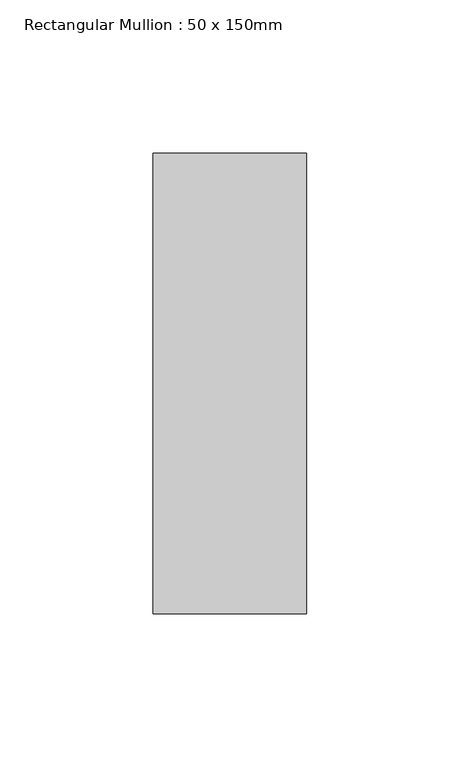
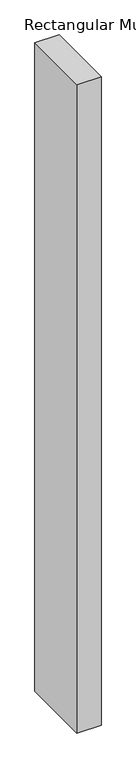
"""IFC4 building model written with IfcOpenShell, lengths in millimetres: member geometry, Rectangular Mullion : 50 x 150mm."""

from ifc_helpers import new_model, si_unit, frame, origin, place, context, project, spatial, polyline, outline, extrude, source, transform, mapped, element, save


def rectangular_mullion_50_x_150mm_a2a5cdf7(model_context):
    return source(origin(), model_context, "Body", "SweptSolid", [
        extrude(outline(polyline([(25.0, 75.0), (25.0, -75.0), (-25.0, -75.0), (-25.0, 75.0), (25.0, 75.0)])), frame((0.0, 0.0, -1416.6666668), z_axis=(0.0, 0.0, 1.0), x_axis=(1.0, 0.0, 0.0)), (0.0, 0.0, 1.0), 1416.6666668),
    ])


if __name__ == "__main__":
    model = new_model("IFC4")
    model_context = context("Model", 3, world=origin())
    ifc_project = project(units=[si_unit("LENGTHUNIT", "METRE", prefix="MILLI")], contexts=[model_context])
    site = spatial("IfcSite", under=ifc_project)
    building = spatial("IfcBuilding", under=site)
    placement = place(None, origin())
    rectangular_mullion_50_x_150mm_shape = rectangular_mullion_50_x_150mm_a2a5cdf7(model_context)
    element("IfcMember", 1, ObjectType="Rectangular Mullion : 50 x 150mm", at=placement, inside=building, context=model_context, shape_type="MappedRepresentation", body=[
        mapped(rectangular_mullion_50_x_150mm_shape, transform((0.0, 0.0, 0.0), x_axis=(1.0, 0.0, 0.0), y_axis=(0.0, 1.0, 0.0), z_axis=(0.0, 0.0, 1.0))),
    ])
    save(model, "model.ifc")

# Revit data of these elements
# Type "Rectangular Mullion : 50 x 150mm"
#   built-in parameter 1007304 = 0.492126 (stored number, unit not read)
#   built-in parameter 1007301 = 0.082021 (stored number, unit not read)
#   built-in parameter 1007300 = 0.082021 (stored number, unit not read)
# Element 1 (IfcMember, "Rectangular Mullion : 50 x 150mm")
#   Materials on its faces: "Aluminium"
# Materials
#   "Aluminium": class "Metal", colour RGB 247 247 247, transparency 0, Description = "Aluminium 6061", Cost = 0
